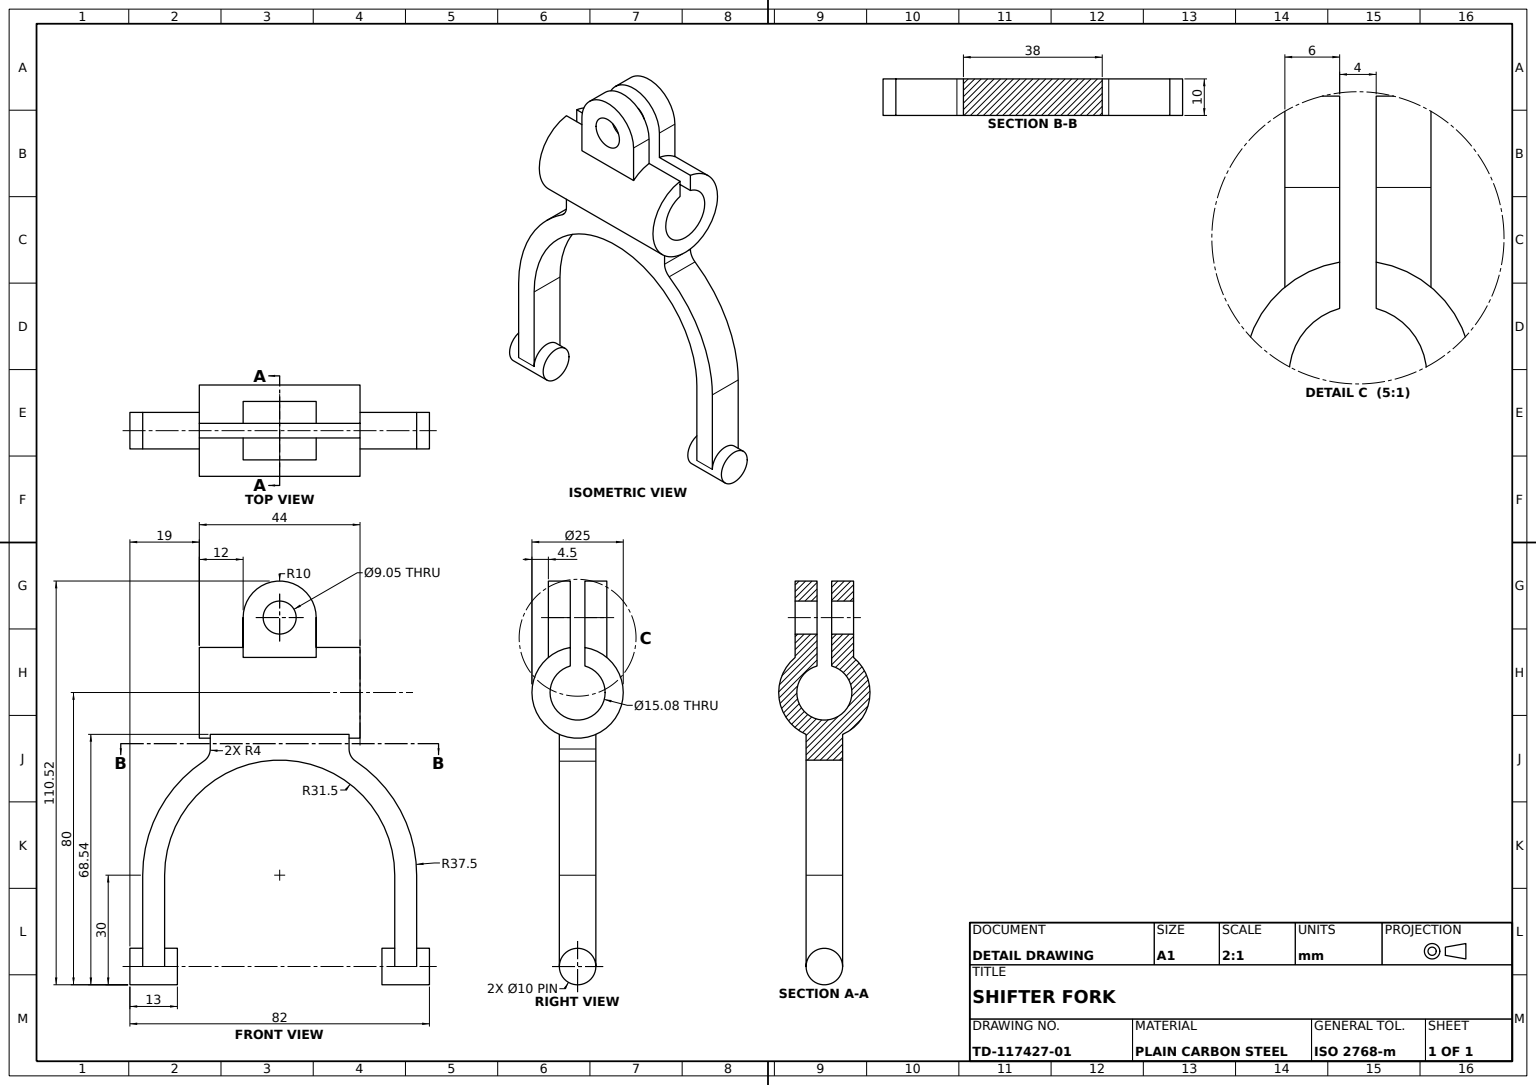
from build123d import *

# Parameters (mm, degrees)
U_FORK_PLATE_DEPTH      = 10
SPLIT_COLLAR_DEPTH      = 22
COLLAR_BORE_SKETCH_R    = 7.54
COLLAR_BORE_DEPTH       = 44
EYE_LUG_FRONT_SKETCH_R  = 4.525
EYE_LUG_FRONT_DEPTH     = 6
EYE_START               = -6
EYE_LUG_REAR_SKETCH_R   = 4.525
EYE_LUG_REAR_DEPTH      = 6
EYE_START_2             = -30
EYE_HOLE_SKETCH_R       = 7.54
EYE_CROSS_HOLE_DEPTH    = 30
FORK_PIN_A_SKETCH_R     = 5
FORK_PIN_A_10_DEPTH     = 6.5
FORK_PIN_B_SKETCH_R     = 5
FORK_PIN_B_10_DEPTH     = 6.5
FORK_EDGE_FILLET_R4_A_R = 4
FORK_EDGE_FILLET_R4_B_R = 4


with BuildPart() as part:
    # U-Fork Profile Sketch → U-Fork Plate (new body)
    with BuildSketch(Plane.XY):
        with BuildLine():
            ThreePointArc((19, -17.667211171), (32.551025104, -31.373310069), (37.504190816, -50))
            Line((37.504190816, -50), (37.504190816, -75))
            Line((37.504190816, -75), (31.504190816, -75))
            Line((31.504190816, -75), (31.504190816, -50))
            ThreePointArc((31.504190816, -50), (0.004190816, -18.5), (-31.495809184, -50))
            Line((-31.495809184, -50), (-31.495809184, -75))
            Line((-31.495809184, -75), (-37.495809184, -75))
            Line((-37.495809184, -75), (-37.495809184, -50))
            ThreePointArc((-37.495809184, -50), (-32.545057682, -31.377529106), (-19, -17.672136918))
            Line((-19, -17.672136918), (-19, 0))
            Line((-19, 0), (19, 0))
            Line((19, 0), (19, -17.667211171))
        make_face()
    extrude(amount=U_FORK_PLATE_DEPTH)

    # Collar Sketch → Split Collar (add, symmetric)
    with BuildSketch(Plane(origin=(0, 0, 0), x_dir=(0, 0, -1), z_dir=(1, 0, 0))):
        with BuildLine():
            Line((-7, 7.269910591), (-7, 12.338962679))
            ThreePointArc((-7, 12.338962679), (-5, -12.5), (-3, 12.338962679))
            Line((-3, 12.338962679), (-3, 7.269910591))
            ThreePointArc((-3, 7.269910591), (-5, -7.54), (-7, 7.269910591))
        make_face()
    extrude(amount=SPLIT_COLLAR_DEPTH, both=True)

    # Collar Bore Sketch → Collar Bore (cut)
    with BuildSketch(Plane(origin=(19, 0, 0), x_dir=(0, 0, -1), z_dir=(1, 0, 0))):
        with Locations((-5, 0)):
            Circle(COLLAR_BORE_SKETCH_R)
    extrude(amount=-COLLAR_BORE_DEPTH, mode=Mode.SUBTRACT)

    # Eye Lug Front Sketch → Eye Lug Front (add)
    with BuildSketch(Plane.XY.offset(7)):
        with BuildLine():
            Line((-10, 5.516178569), (10, 5.516178569))
            Line((10, 5.516178569), (10, 20.516178569))
            ThreePointArc((10, 20.516178569), (0, 30.516178569), (-10, 20.516178569))
            Line((-10, 20.516178569), (-10, 5.516178569))
        make_face()
        with Locations((0, 20.516178569)):
            Circle(EYE_LUG_FRONT_SKETCH_R, mode=Mode.SUBTRACT)
    extrude(amount=EYE_LUG_FRONT_DEPTH)

    # Eye Lug Rear Sketch → Eye Lug Rear (add)
    with BuildSketch(Plane.XY.offset(3).offset(EYE_START)):
        with BuildLine():
            Line((10, 20.516178569), (10, 5.516178569))
            Line((10, 5.516178569), (-10, 5.516178569))
            Line((-10, 5.516178569), (-10, 20.516178569))
            ThreePointArc((-10, 20.516178569), (0, 30.516178569), (10, 20.516178569))
        make_face()
        with Locations((0, 20.516178569)):
            Circle(EYE_LUG_REAR_SKETCH_R, mode=Mode.SUBTRACT)
    extrude(amount=EYE_LUG_REAR_DEPTH)

    # Eye Hole Sketch → Eye Cross Hole (cut)
    with BuildSketch(Plane.ZY.offset(10).offset(EYE_START_2)):
        with Locations((5, 0)):
            Circle(EYE_HOLE_SKETCH_R)
    extrude(amount=EYE_CROSS_HOLE_DEPTH, mode=Mode.SUBTRACT)

    # Fork Pin A Sketch → Fork Pin A Ø10 (add, symmetric)
    with BuildSketch(Plane(origin=(34.5, 0, 0), x_dir=(0, 0, -1), z_dir=(1, 0, 0))):
        with Locations((-5, -75)):
            Circle(FORK_PIN_A_SKETCH_R)
    extrude(amount=FORK_PIN_A_10_DEPTH, both=True)

    # Fork Pin B Sketch → Fork Pin B Ø10 (add, symmetric)
    with BuildSketch(Plane(origin=(-34.5, 0, 0), x_dir=(0, 0, -1), z_dir=(1, 0, 0))):
        with Locations((-5, -75)):
            Circle(FORK_PIN_B_SKETCH_R)
    extrude(amount=FORK_PIN_B_10_DEPTH, both=True)

    # Fork Edge Fillet R4 A
    fork_edge_fillet_r4_a_edges = [part.edges().sort_by_distance(p)[0] for p in [
        (19, -17.667211171, 5),
    ]]
    fillet(fork_edge_fillet_r4_a_edges, radius=FORK_EDGE_FILLET_R4_A_R)

    # Fork Edge Fillet R4 B
    fork_edge_fillet_r4_b_edges = [part.edges().sort_by_distance(p)[0] for p in [
        (-19, -17.672136918, 5),
    ]]
    fillet(fork_edge_fillet_r4_b_edges, radius=FORK_EDGE_FILLET_R4_B_R)


solid = part.part
